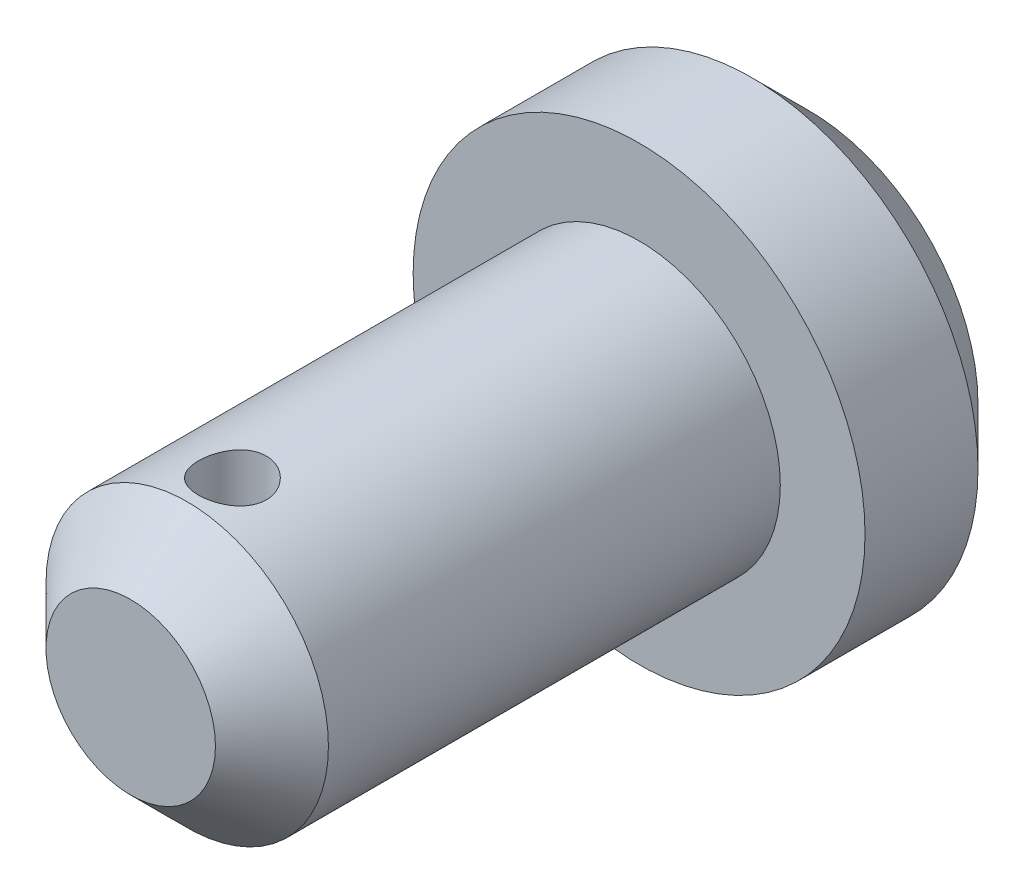
from build123d import *

# Parameters (mm, degrees)
HEAD_AND_SHANK_PROFILE_80_50_R   = 40
HEAD_AND_SHANK_PROFILE_80_50_R_2 = 25
HEAD_80_DEPTH                    = 30
SKETCH1_3_R                      = 25
SHANK_50_DEPTH                   = 120
HEAD_CHAMFER_10X45_SIZE          = 10
SHANK_END_CHAMFER_10X45_SIZE     = 10
CROSS_HOLE_PROFILE_R             = 6
CROSS_HOLE_12_DEPTH              = 30


with BuildPart() as part:
    # Head and Shank Profile _80-_50 → Head _80 (new body)
    # profile 1 of 2: a face of its own
    with BuildSketch(Plane.XY):
        Circle(HEAD_AND_SHANK_PROFILE_80_50_R)
        Circle(HEAD_AND_SHANK_PROFILE_80_50_R_2, mode=Mode.SUBTRACT)
    # profile 2 of 2: a face of its own
    with BuildSketch(Plane.XY):
        Circle(HEAD_AND_SHANK_PROFILE_80_50_R_2)
    extrude(amount=HEAD_80_DEPTH)

    # Sketch1_3 → Shank _50 (add)
    with BuildSketch(Plane.XY):
        with Locations(Location((0, 0, 0), (0, 0, 180))):
            Circle(SKETCH1_3_R)
    extrude(amount=SHANK_50_DEPTH)

    # Head Chamfer 10x45
    head_chamfer_10x45_edges = [part.edges().sort_by_distance(p)[0] for p in [
        (-40, 0, 0),
    ]]
    chamfer(head_chamfer_10x45_edges, length=HEAD_CHAMFER_10X45_SIZE)

    # Shank End Chamfer 10x45
    shank_end_chamfer_10x45_edges = [part.edges().sort_by_distance(p)[0] for p in [
        (25, 0, 120),
    ]]
    chamfer(shank_end_chamfer_10x45_edges, length=SHANK_END_CHAMFER_10X45_SIZE)

    # Cross Hole Profile → Cross Hole _12 (cut, symmetric)
    with BuildSketch(Plane(origin=(0, 0, 0), x_dir=(1, 0, 0), z_dir=(0, 1, 0))):
        with Locations(Location((0, -102, 0), (0, 0, 270))):
            Circle(CROSS_HOLE_PROFILE_R)
    extrude(amount=CROSS_HOLE_12_DEPTH, both=True, mode=Mode.SUBTRACT)


solid = part.part
